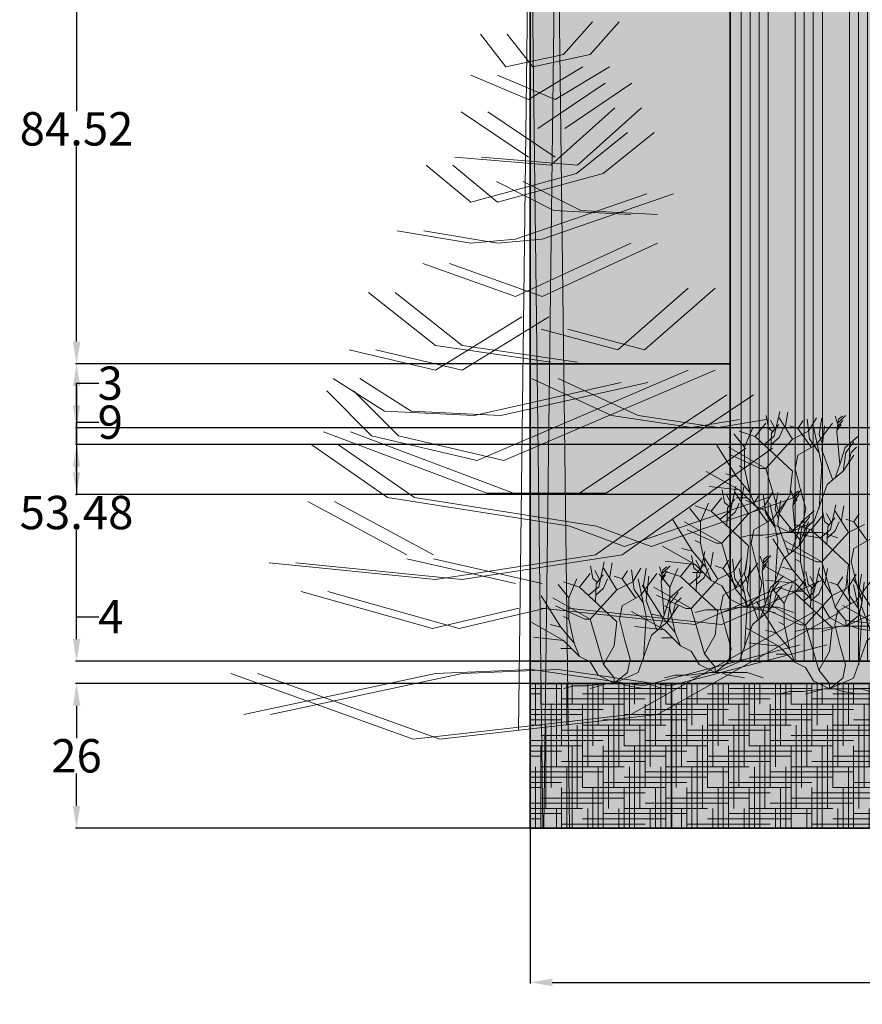
# Model space of a CAD drawing. Units: inches. Extents: x 221 to 874, y 171 to 738.
# Tile 1 of 11: x 221 to 373, y 171 to 348. Entities that reach past the tile are written whole.
import ezdxf

# ---------------------------------------------------------------- set-up
doc = ezdxf.new("R2010")
doc.units = ezdxf.units.IN
doc.header["$MEASUREMENT"] = 0
for name, color, linetype, lineweight in [('A-ANNO-DIMS', 2, 'Continuous', 18), ('A-ELEV', 7, 'Continuous', 35), ('A-ELEV-PATT', 8, 'Continuous', 13), ('L-PLNT', 3, 'Continuous', 13)]:
    doc.layers.add(name, color=color, linetype=linetype, lineweight=lineweight)
doc.styles.get("Standard").update_dxf_attribs({"font": 'arial.ttf'})
doc.dimstyles.get("Standard").update_dxf_attribs({"dimtxt": 6, "dimasz": 4, "dimexe": 0.18, "dimexo": 0.0625, "dimgap": 0.09, "dimtad": 0, "dimtih": 1, "dimtoh": 1, "dimdec": 0, "dimzin": 0, "dimdsep": 46, "dimlunit": 3, "dimtxsty": 'Standard', "dimcen": 0.09, "dimadec": 0, "dimazin": 0, "dimtfac": 1, "dimtdec": 0, "dimtofl": 0, "dimtmove": 0, "dimatfit": 3, "dimfxl": 1, "dimtolj": 1, "dimtzin": 0, "dimarcsym": 0})

# ---------------------------------------------------------------- blocks, each defined once
blk = doc.blocks.new('SHRUB-A')
for p, q in [((15.5, 17.76), (13.1, 21.6)), ((18.38, 19.2), (19.82, 21.6)), ((6.86, 16.32), (8.3, 19.68)), ((8.78, 18.24), (10.7, 20.64)), ((19.82, 16.8), (22.7, 20.64)), ((6.86, 16.32), (4.94, 18.72)), ((8.78, 18.24), (5.9, 19.2)), ((15.5, 12), (8.78, 18.24)), ((10.7, 12.48), (15.5, 17.76)), ((15.5, 17.76), (18.38, 19.2)), ((5.42, 11.04), (1.91, 16.66)), ((10.7, 12.48), (3.98, 16.32)), ((6.86, 12.48), (6.86, 16.32)), ((16.46, 14.88), (19.82, 16.8)), ((25.1, 15.36), (26.54, 17.28)), ((9.74, 12.48), (4.46, 14.88)), ((15.98, 12.48), (16.46, 14.88)), ((24.62, 12), (25.1, 15.36)), ((24.62, 12), (26.54, 14.88)), ((6.86, 12.48), (5.9, 12.96)), ((7.82, 8.16), (6.86, 12.48)), ((10.7, 12.48), (9.74, 12.48)), ((13.1, 4.32), (10.7, 12.48)), ((16.94, 8.64), (15.98, 12.48)), ((5.9, 8.64), (0, 11.96)), ((5.42, 11.04), (3.5, 11.52)), ((7.82, 8.16), (5.42, 11.04)), ((15.02, 7.68), (15.5, 12)), ((21.74, 9.6), (24.62, 12)), ((5.9, 8.64), (0.53, 9.22)), ((19.34, 2.88), (21.74, 9.6)), ((8.78, 5.76), (5.9, 8.64)), ((8.78, 5.76), (7.82, 8.16)), ((13.1, 4.32), (15.02, 7.68)), ((17.9, 5.28), (16.94, 8.64)), ((10.7, 4.8), (8.78, 5.76)), ((12.14, 2.4), (10.7, 4.8)), ((15.02, 1.92), (13.1, 4.32)), ((17.42, 2.88), (17.9, 5.28)), ((15.02, 0.96), (12.14, 2.4)), ((15.02, 0.96), (19.34, 2.88)), ((15.02, 0.96), (17.42, 2.88)), ((15.02, 0.96), (15.02, 1.92)), ((15.02, 0.96), (20.78, 0.96)), ((20.78, 0.96), (23.66, 0))]:
    blk.add_line(p, q)
blk = doc.blocks.new('GRASS-TUFT')
for p, q in [((0.58, 10.54), (1.31, 11.09)), ((0.28, 8.35), (0.58, 10.54)), ((0.83, 2.4), (0.28, 8.35)), ((1.8, 5.45), (4.12, 7.49)), ((0.83, 2.4), (1.8, 5.45)), ((0, 0), (0.83, 2.4))]:
    blk.add_line(p, q)
blk = doc.blocks.new('GRASS-SPRIG')
for p, q in [((1.44, 3.36), (0, 3.84)), ((1.44, 3.36), (2.4, 4.8)), ((3.84, 0), (1.44, 3.36))]:
    blk.add_line(p, q)
blk = doc.blocks.new('*D20')
at = {"layer": 'A-ANNO-DIMS', "color": 0, "lineweight": -2, "transparency": 16777216}
for p, q in [((313.08, 202.65), (313.08, 174.79)), ((805.08, 202.65), (805.08, 174.79)), ((317.08, 174.97), (552.27, 174.97)), ((801.08, 174.97), (565.89, 174.97))]:
    blk.add_line(p, q, dxfattribs=at)
at = {"layer": 'A-ANNO-DIMS', "color": 0, "transparency": 16777216}
for points in [[(317.08, 175.63), (317.08, 174.3), (313.08, 174.97)], [(801.08, 175.63), (801.08, 174.3), (805.08, 174.97)]]:
    blk.add_solid(points, dxfattribs=at)
at = {"layer": 'Defpoints', "color": 0, "transparency": 16777216}
for p in [(313.08, 202.72), (805.08, 202.72), (805.08, 174.97)]:
    blk.add_point(p, dxfattribs=at)
at = {"layer": 'A-ANNO-DIMS', "color": 0, "transparency": 16777216, "insert": (559.08, 174.97), "char_height": 6, "attachment_point": 5}
blk.add_mtext('\\A1;492', dxfattribs=at)
blk = doc.blocks.new('*D29')
at = {"layer": 'A-ANNO-DIMS', "color": 0, "lineweight": -2, "transparency": 16777216}
for p, q in [((313.02, 228.72), (231.36, 228.72)), ((231.54, 224.72), (231.54, 218.87)), ((231.54, 206.72), (231.54, 212.56)), ((313.02, 202.72), (231.36, 202.72))]:
    blk.add_line(p, q, dxfattribs=at)
at = {"layer": 'A-ANNO-DIMS', "color": 0, "transparency": 16777216}
for points in [[(230.88, 224.72), (232.21, 224.72), (231.54, 228.72)], [(230.88, 206.72), (232.21, 206.72), (231.54, 202.72)]]:
    blk.add_solid(points, dxfattribs=at)
at = {"layer": 'Defpoints', "color": 0, "transparency": 16777216}
for p in [(231.54, 228.72), (313.08, 228.72), (313.08, 202.72)]:
    blk.add_point(p, dxfattribs=at)
at = {"layer": 'A-ANNO-DIMS', "color": 0, "transparency": 16777216, "insert": (231.54, 215.72), "char_height": 6, "attachment_point": 5}
blk.add_mtext('\\A1;26', dxfattribs=at)
blk = doc.blocks.new('*D30')
at = {"layer": 'A-ANNO-DIMS', "color": 0, "lineweight": -2, "transparency": 16777216}
for p, q in [((231.54, 236.72), (231.54, 240.72)), ((231.54, 240.72), (235.54, 240.72)), ((313.02, 232.72), (231.36, 232.72)), ((313.02, 228.72), (231.36, 228.72)), ((231.54, 224.72), (231.54, 220.72))]:
    blk.add_line(p, q, dxfattribs=at)
at = {"layer": 'A-ANNO-DIMS', "color": 0, "transparency": 16777216}
for points in [[(230.88, 236.72), (232.21, 236.72), (231.54, 232.72)], [(230.88, 224.72), (232.21, 224.72), (231.54, 228.72)]]:
    blk.add_solid(points, dxfattribs=at)
at = {"layer": 'Defpoints', "color": 0, "transparency": 16777216}
for p in [(231.54, 232.72), (313.08, 232.72), (313.08, 228.72)]:
    blk.add_point(p, dxfattribs=at)
at = {"layer": 'A-ANNO-DIMS', "color": 0, "transparency": 16777216, "insert": (237.71, 240.72), "char_height": 6, "attachment_point": 5}
blk.add_mtext('\\A1;4', dxfattribs=at)
blk = doc.blocks.new('*D31')
at = {"layer": 'A-ANNO-DIMS', "color": 0, "lineweight": -2, "transparency": 16777216}
for p, q in [((313.02, 286.2), (231.36, 286.2)), ((231.54, 282.2), (231.54, 262.61)), ((231.54, 236.72), (231.54, 256.3)), ((313.02, 232.72), (231.36, 232.72))]:
    blk.add_line(p, q, dxfattribs=at)
at = {"layer": 'A-ANNO-DIMS', "color": 0, "transparency": 16777216}
for points in [[(230.88, 282.2), (232.21, 282.2), (231.54, 286.2)], [(230.88, 236.72), (232.21, 236.72), (231.54, 232.72)]]:
    blk.add_solid(points, dxfattribs=at)
at = {"layer": 'Defpoints', "color": 0, "transparency": 16777216}
for p in [(231.54, 286.2), (313.08, 286.2), (313.08, 232.72)]:
    blk.add_point(p, dxfattribs=at)
at = {"layer": 'A-ANNO-DIMS', "color": 0, "transparency": 16777216, "insert": (231.54, 259.46), "char_height": 6, "attachment_point": 5}
blk.add_mtext('\\A1;53.48', dxfattribs=at)
blk = doc.blocks.new('*D32')
at = {"layer": 'A-ANNO-DIMS', "color": 0, "lineweight": -2, "transparency": 16777216}
for p, q in [((313.02, 370.72), (231.36, 370.72)), ((231.54, 366.72), (231.54, 331.61)), ((231.54, 290.2), (231.54, 325.3)), ((313.02, 286.2), (231.36, 286.2))]:
    blk.add_line(p, q, dxfattribs=at)
at = {"layer": 'A-ANNO-DIMS', "color": 0, "transparency": 16777216}
for points in [[(230.88, 366.72), (232.21, 366.72), (231.54, 370.72)], [(230.88, 290.2), (232.21, 290.2), (231.54, 286.2)]]:
    blk.add_solid(points, dxfattribs=at)
at = {"layer": 'Defpoints', "color": 0, "transparency": 16777216}
for p in [(231.54, 370.72), (313.08, 370.72), (313.08, 286.2)]:
    blk.add_point(p, dxfattribs=at)
at = {"layer": 'A-ANNO-DIMS', "color": 0, "transparency": 16777216, "insert": (231.54, 328.46), "char_height": 6, "attachment_point": 5}
blk.add_mtext('\\A1;84.52', dxfattribs=at)
blk = doc.blocks.new('*D67')
at = {"layer": 'A-ANNO-DIMS', "color": 0, "lineweight": -2, "transparency": 16777216}
for p, q in [((231.54, 271.72), (231.54, 275.72)), ((231.54, 275.72), (235.54, 275.72)), ((541.02, 271.72), (231.36, 271.72)), ((231.54, 266.72), (231.54, 267.72)), ((541.02, 262.72), (231.36, 262.72))]:
    blk.add_line(p, q, dxfattribs=at)
at = {"layer": 'A-ANNO-DIMS', "color": 0, "transparency": 16777216}
for points in [[(230.88, 267.72), (232.21, 267.72), (231.54, 271.72)], [(230.88, 266.72), (232.21, 266.72), (231.54, 262.72)]]:
    blk.add_solid(points, dxfattribs=at)
at = {"layer": 'Defpoints', "color": 0, "transparency": 16777216}
for p in [(231.54, 271.72), (541.08, 271.72), (541.08, 262.72)]:
    blk.add_point(p, dxfattribs=at)
at = {"layer": 'A-ANNO-DIMS', "color": 0, "transparency": 16777216, "insert": (237.61, 275.72), "char_height": 6, "attachment_point": 5}
blk.add_mtext('\\A1;9', dxfattribs=at)
blk = doc.blocks.new('*D68')
at = {"layer": 'A-ANNO-DIMS', "color": 0, "lineweight": -2, "transparency": 16777216}
for p, q in [((231.54, 278.72), (231.54, 282.72)), ((231.54, 282.72), (235.54, 282.72)), ((541.02, 274.72), (231.36, 274.72)), ((541.02, 271.72), (231.36, 271.72)), ((231.54, 267.72), (231.54, 263.72))]:
    blk.add_line(p, q, dxfattribs=at)
at = {"layer": 'A-ANNO-DIMS', "color": 0, "transparency": 16777216}
for points in [[(230.88, 278.72), (232.21, 278.72), (231.54, 274.72)], [(230.88, 267.72), (232.21, 267.72), (231.54, 271.72)]]:
    blk.add_solid(points, dxfattribs=at)
at = {"layer": 'Defpoints', "color": 0, "transparency": 16777216}
for p in [(231.54, 274.72), (541.08, 274.72), (541.08, 271.72)]:
    blk.add_point(p, dxfattribs=at)
at = {"layer": 'A-ANNO-DIMS', "color": 0, "transparency": 16777216, "insert": (237.6, 282.72), "char_height": 6, "attachment_point": 5}
blk.add_mtext('\\A1;3', dxfattribs=at)

msp = doc.modelspace()

# ---------------------------------------------------------------- hatches: boundary and pattern name
at = {"layer": 'A-ELEV-PATT'}
h = msp.add_hatch(color=256, dxfattribs=at)
h.dxf.hatch_style = 1
h.paths.add_polyline_path([(349.0786, 286.1996), (313.0786, 286.1996), (313.0786, 232.7164), (349.0786, 232.7164)])
h.paths.add_polyline_path([(464.0786, 286.1996), (406.0786, 286.1996), (406.0786, 232.7164), (464.0786, 232.7164)])
h.paths.add_polyline_path([(541.0786, 286.1996), (493.0786, 286.1996), (493.0786, 232.7164), (541.0786, 232.7164)])
h.paths.add_polyline_path([(541.0786, 370.7164), (493.0786, 370.7164), (493.0786, 286.1996), (541.0786, 286.1996)])
h.paths.add_polyline_path([(464.0786, 370.7164), (406.0786, 370.7164), (406.0786, 286.1996), (464.0786, 286.1996)])
h.paths.add_polyline_path([(349.0786, 370.7164), (313.0786, 370.7164), (313.0786, 286.1996), (349.0786, 286.1996)])
h.paths.add_polyline_path([(349.0786, 454.7164), (313.0786, 454.7164), (313.0786, 370.7164), (349.0786, 370.7164)])
h.paths.add_polyline_path([(464.0786, 454.7164), (406.0786, 454.7164), (406.0786, 370.7164), (464.0786, 370.7164)])
h.paths.add_polyline_path([(541.0786, 418.7164), (541.0786, 454.7164), (493.0786, 454.7164), (493.0786, 370.7164), (541.0786, 370.7164)])
h.paths.add_polyline_path([(541.0786, 550.7164), (493.0786, 550.7164), (493.0786, 454.7164), (541.0786, 454.7164)])
h.paths.add_polyline_path([(464.0786, 550.7164), (406.0786, 550.7164), (406.0786, 454.7164), (464.0786, 454.7164)])
h.paths.add_polyline_path([(349.0786, 550.7164), (313.0786, 550.7164), (313.0786, 454.7164), (349.0786, 454.7164)])
h.paths.add_polyline_path([(349.0786, 586.7164), (313.0786, 586.7164), (313.0786, 550.7164), (349.0786, 550.7164)])
h.paths.add_polyline_path([(464.0786, 586.7164), (406.0786, 586.7164), (406.0786, 550.7164), (464.0786, 550.7164)])
h.paths.add_polyline_path([(541.0786, 574.7164), (541.0786, 586.7164), (493.0786, 586.7164), (493.0786, 550.7164), (541.0786, 550.7164)])
h.paths.add_polyline_path([(541.0786, 670.7164), (493.0786, 670.7164), (493.0786, 586.7164), (541.0786, 586.7164)])
h.paths.add_polyline_path([(464.0786, 670.7164), (406.0786, 670.7164), (406.0786, 586.7164), (464.0786, 586.7164)])
h.paths.add_polyline_path([(349.0786, 670.7164), (313.0786, 670.7164), (313.0786, 586.7164), (349.0786, 586.7164)])
h.paths.add_polyline_path([(406.0786, 706.7164), (313.0786, 706.7164), (313.0786, 670.7164), (349.0786, 670.7164), (406.0786, 670.7164)])
h.paths.add_polyline_path([(464.0786, 706.7164), (406.0786, 706.7164), (406.0786, 670.7164), (464.0786, 670.7164)])
h.paths.add_polyline_path([(541.0786, 706.7164), (493.0786, 706.7164), (493.0786, 688.7164), (493.0786, 670.7164), (541.0786, 670.7164)])
h.paths.add_polyline_path([(660.0786, 610.7164), (541.0786, 610.7164), (541.0786, 586.7164), (541.0786, 574.7164), (660.0786, 574.7164)])
h.paths.add_polyline_path([(781.0786, 610.7164), (660.0786, 610.7164), (660.0786, 574.7164), (769.0786, 574.7164), (781.0786, 574.7164)])
h.paths.add_polyline_path([(781.0786, 574.7164), (769.0786, 574.7164), (769.0786, 476.1199), (781.0786, 476.1199)])
h.paths.add_polyline_path([(781.0786, 476.1199), (769.0786, 476.1199), (769.0786, 457.7164), (781.0786, 457.7164)])
h.paths.add_polyline_path([(781.0786, 377.1023), (705.9097, 377.1023), (705.9097, 286.1996), (781.0786, 286.1996)])
h.paths.add_polyline_path([(741.9618, 338.8486), (756.9618, 338.8486), (756.9618, 329.8486), (741.9618, 329.8486)], flags=16)
h.paths.add_polyline_path([(648.9097, 377.1023), (598.0786, 377.1023), (598.0786, 286.1996), (648.9097, 286.1996)])
h.paths.add_polyline_path([(781.0786, 286.1996), (705.9097, 286.1996), (705.9097, 280.7164), (648.9097, 280.7164), (648.9097, 286.1996), (598.0786, 286.1996), (598.0786, 280.7164), (550.0786, 280.7164), (550.0786, 286.1996), (541.0786, 286.1996), (541.0786, 274.7164), (781.0786, 274.7164)])
h.paths.add_polyline_path([(660.0786, 562.7164), (546.3477, 562.7164), (546.3477, 457.7164), (660.0786, 457.7164)])
h = msp.add_hatch(color=256, dxfattribs=at)
h.paths.add_polyline_path([(406.0786, 670.7164), (349.0786, 670.7164), (349.0786, 454.7164), (406.0786, 454.7164)])
h.paths.add_polyline_path([(406.0786, 454.7164), (349.0786, 454.7164), (349.0786, 232.7164), (406.0786, 232.7164)])
h = msp.add_hatch(dxfattribs=at)
h.set_pattern_fill('ANSI34', color=256, scale=13, angle=45, style=0)
h.paths.add_polyline_path([(406.0786, 670.7164), (349.0786, 670.7164), (349.0786, 454.7164), (406.0786, 454.7164)])
h.paths.add_polyline_path([(406.0786, 454.7164), (349.0786, 454.7164), (349.0786, 232.7164), (406.0786, 232.7164)])
msp.add_hatch(color=256, dxfattribs=at).paths.add_polyline_path([(313.0786, 232.7164), (313.0786, 228.7164), (541.0786, 228.7164), (541.0786, 232.7164)])
h = msp.add_hatch(color=256, dxfattribs=at)
h.set_gradient(color1=(99, 100, 102), color2=(91, 91, 91), rotation=180, name='INVCURVED')
h.paths.add_polyline_path([(338.5139, 202.7164), (338.5139, 228.7164), (313.0786, 228.7164), (313.0786, 202.7164)])
h = msp.add_hatch(dxfattribs=at)
h.set_pattern_fill('HOUND', color=256, scale=15, style=0)
h.paths.add_polyline_path([(338.5139, 228.7164), (313.0786, 228.7164), (313.0786, 202.7164), (338.5139, 202.7164)])
h = msp.add_hatch(color=256, dxfattribs=at)
h.set_gradient(color1=(147, 149, 152), color2=(91, 91, 91), name='CURVED')
h.paths.add_polyline_path([(384.2386, 202.7164), (384.2386, 228.7164), (338.5139, 228.7164), (338.5139, 202.7164)])
h = msp.add_hatch(dxfattribs=at)
h.set_pattern_fill('HOUND', color=256, scale=15, style=0)
h.paths.add_polyline_path([(384.2386, 228.7164), (338.5139, 228.7164), (338.5139, 202.7164), (384.2386, 202.7164)])

# ---------------------------------------------------------------- linework, layer by layer
at = {"layer": 'A-ELEV'}
for p, q in [((313.0786, 232.7164), (313.0786, 706.7164)), ((349.0786, 232.7164), (349.0786, 670.7164)), ((313.0786, 286.1996), (349.0786, 286.1996)), ((541.0786, 232.7164), (313.0786, 232.7164)), ((313.0786, 232.7164), (313.0786, 228.7164)), ((541.0786, 228.7164), (313.0786, 228.7164)), ((313.0786, 228.7164), (313.0786, 202.7164)), ((338.5139, 228.7164), (338.5139, 202.7164)), ((805.0786, 202.7164), (313.0786, 202.7164))]:
    msp.add_line(p, q, dxfattribs=at)
at = {"layer": 'L-PLNT'}
for p, q in [((313.0656, 386.0299), (310.9947, 220.2893)), ((313.0656, 386.0299), (315.358, 202.7164)), ((317.8656, 386.0299), (315.5752, 202.7164)), ((317.8656, 386.0299), (320.158, 202.7164)), ((355.9588, 274.6734), (355.5318, 276.9424)), ((356.9968, 273.1874), (357.9728, 277.6474)), ((360.2698, 272.6584), (357.8698, 276.4984)), ((358.9498, 274.6734), (359.4378, 277.4904)), ((363.3438, 272.6394), (362.9168, 276.2384)), ((363.1498, 274.0984), (364.5898, 276.4984)), ((365.0528, 273.5004), (365.5418, 276.4734)), ((367.9218, 276.7864), (368.3488, 275.4564)), ((368.4708, 275.6124), (369.8138, 276.9424)), ((351.6298, 271.2184), (353.0698, 274.5784)), ((353.5498, 273.1384), (355.4698, 275.5384)), ((356.7528, 273.9694), (355.9588, 274.6734)), ((357.1498, 274.5174), (356.3258, 276.0824)), ((356.5088, 273.7344), (357.7898, 275.2994)), ((357.8508, 272.9524), (358.5838, 274.5954)), ((365.5498, 267.8584), (364.1098, 274.5784)), ((364.5898, 271.6984), (367.4698, 275.5384)), ((365.5498, 270.7384), (366.0298, 275.0584)), ((368.2878, 274.2824), (369.0198, 275.2994)), ((368.4098, 274.9084), (369.3258, 276.0034)), ((351.6298, 271.2184), (349.7098, 273.6184)), ((353.5498, 273.1384), (350.6698, 274.0984)), ((360.2698, 266.8984), (353.5498, 273.1384)), ((355.1048, 271.6224), (356.9968, 273.1874)), ((356.3868, 270.5264), (356.5088, 273.7344)), ((356.4478, 271.7004), (357.8508, 272.9524)), ((360.2698, 272.6584), (363.1498, 274.0984)), ((365.0528, 270.2134), (363.3438, 272.7174)), ((365.6638, 271.7004), (365.0528, 273.5004)), ((350.1898, 265.9384), (346.6748, 271.5534)), ((355.4698, 267.3784), (348.7498, 271.2184)), ((351.6298, 267.3784), (351.6298, 271.2184)), ((355.4698, 267.3784), (360.2698, 272.6584)), ((361.2298, 269.7784), (364.5898, 271.6984)), ((369.8698, 270.2584), (371.3098, 272.1784)), ((370.8298, 270.2584), (371.7898, 271.2184)), ((354.5098, 267.3784), (349.2298, 269.7784)), ((360.7498, 267.3784), (361.2298, 269.7784)), ((367.4698, 265.4584), (365.5498, 270.7384)), ((369.3898, 266.8984), (369.8698, 270.2584)), ((369.3898, 266.8984), (371.3098, 269.7784)), ((370.3498, 268.3384), (370.8298, 270.2584)), ((351.6298, 267.3784), (350.6698, 267.8584)), ((352.5898, 263.0584), (351.6298, 267.3784)), ((355.4698, 267.3784), (354.5098, 267.3784)), ((357.8698, 259.2184), (355.4698, 267.3784)), ((361.7098, 263.5384), (360.7498, 267.3784)), ((365.0698, 260.1784), (365.5498, 267.8584)), ((350.6698, 263.5384), (344.7668, 266.8594)), ((350.1898, 265.9384), (348.2698, 266.4184)), ((352.5898, 263.0584), (350.1898, 265.9384)), ((359.7898, 262.5784), (360.2698, 266.8984)), ((366.5098, 264.4984), (369.3898, 266.8984)), ((350.6698, 263.5384), (345.3018, 264.1204)), ((349.0936, 259.7609), (350.0696, 264.2209)), ((351.0466, 261.2469), (351.5346, 264.0639)), ((364.1098, 257.7784), (366.5098, 264.4984)), ((348.0556, 261.2469), (347.6286, 263.5159)), ((349.2466, 261.0909), (348.4226, 262.6559)), ((352.1098, 262.0984), (350.1898, 262.0984)), ((353.5498, 260.6584), (350.6698, 263.5384)), ((353.5498, 260.6584), (352.5898, 263.0584)), ((355.4406, 259.2129), (355.0136, 262.8119)), ((357.1496, 260.0739), (357.6386, 263.0469)), ((357.8698, 259.2184), (359.7898, 262.5784)), ((360.0186, 263.3599), (360.4456, 262.0299)), ((360.5066, 261.4819), (361.4226, 262.5769)), ((360.5676, 262.1859), (361.9106, 263.5159)), ((362.6698, 260.1784), (361.7098, 263.5384)), ((273.0956, 261.4559), (290.9246, 251.8709)), ((277.8956, 261.4559), (295.7246, 251.8709)), ((348.8496, 260.5429), (348.0556, 261.2469)), ((348.4836, 257.0999), (348.6056, 260.3079)), ((348.6056, 260.3079), (349.8866, 261.8729)), ((349.9476, 259.5259), (350.6806, 261.1689)), ((355.4698, 259.6984), (353.5498, 260.6584)), ((357.6466, 254.4319), (356.2066, 261.1519)), ((357.6466, 257.3119), (358.1266, 261.6319)), ((360.3846, 260.8559), (361.1166, 261.8729)), ((367.0768, 256.3874), (368.0528, 260.8474)), ((369.0298, 257.8734), (369.5178, 260.6904)), ((347.2016, 258.1959), (349.0936, 259.7609)), ((348.5446, 258.2739), (349.9476, 259.5259)), ((357.1496, 256.7869), (355.4406, 259.2909)), ((356.9098, 257.2984), (355.4698, 259.6984)), ((357.7606, 258.2739), (357.1496, 260.0739)), ((359.7898, 256.8184), (357.8698, 259.2184)), ((362.1898, 257.7784), (362.6698, 260.1784)), ((363.6298, 256.3384), (365.5498, 258.7384)), ((366.0388, 257.8734), (365.6118, 260.1424)), ((367.2298, 257.7174), (366.4058, 259.2824)), ((370.3498, 255.8584), (367.9498, 259.6984)), ((359.7898, 255.8584), (356.9098, 257.2984)), ((359.5666, 252.0319), (357.6466, 257.3119)), ((359.7898, 255.8584), (364.1098, 257.7784)), ((359.7898, 255.8584), (362.1898, 257.7784)), ((361.7098, 254.4184), (359.7898, 256.8184)), ((359.7898, 255.8584), (359.7898, 256.8184)), ((363.6298, 256.3384), (360.7498, 257.2984)), ((361.7098, 254.4184), (363.1498, 257.7784)), ((362.4466, 254.9119), (362.9266, 256.8319)), ((362.9266, 256.8319), (363.8866, 257.7919)), ((366.8328, 257.1694), (366.0388, 257.8734)), ((366.4668, 253.7264), (366.5888, 256.9344)), ((366.5888, 256.9344), (367.8698, 258.4994)), ((367.9308, 256.1524), (368.6638, 257.7954)), ((370.3498, 255.8584), (373.2298, 257.2984)), ((352.5898, 255.3784), (350.6698, 254.8984)), ((354.9898, 255.3784), (352.5898, 255.3784)), ((358.8298, 255.8584), (354.9898, 255.3784)), ((358.8298, 255.8584), (355.4698, 254.8984)), ((358.8298, 255.8584), (360.7498, 255.8584)), ((359.7898, 255.8584), (365.5498, 255.8584)), ((360.7498, 255.8584), (362.1898, 255.3784)), ((362.1898, 255.3784), (365.0698, 254.8984)), ((370.3498, 250.0984), (363.6298, 256.3384)), ((365.1848, 254.8224), (367.0768, 256.3874)), ((365.5498, 250.5784), (370.3498, 255.8584)), ((365.5498, 255.8584), (368.4298, 254.8984)), ((366.5278, 254.9004), (367.9308, 256.1524)), ((360.2698, 249.1384), (356.7548, 254.7534)), ((357.1666, 246.7519), (357.6466, 254.4319)), ((365.5498, 250.5784), (358.8298, 254.4184)), ((361.7098, 250.5784), (361.7098, 254.4184)), ((371.3098, 252.9784), (374.6698, 254.8984)), ((342.5149, 249.4974), (342.0879, 251.7664)), ((343.5529, 248.0114), (344.5289, 252.4714)), ((345.5059, 249.4974), (345.9939, 252.3144)), ((354.4779, 251.6104), (354.9049, 250.2804)), ((355.0269, 250.4364), (356.3699, 251.7664)), ((364.5898, 250.5784), (359.3098, 252.9784)), ((370.8298, 250.5784), (371.3098, 252.9784)), ((290.9246, 251.1339), (310.4786, 246.7099)), ((295.7246, 251.1339), (315.2786, 246.7099)), ((324.3871, 247.6064), (323.9601, 249.8754)), ((325.4251, 246.1204), (326.4011, 250.5804)), ((327.3781, 247.6064), (327.8661, 250.4234)), ((336.3501, 249.7194), (336.7771, 248.3894)), ((336.8991, 248.5454), (338.2421, 249.8754)), ((343.7059, 249.3414), (342.8819, 250.9064)), ((343.0649, 248.5584), (344.3459, 250.1234)), ((349.8999, 247.4634), (349.4729, 251.0624)), ((351.6089, 248.3244), (352.0979, 251.2974)), ((352.1059, 245.5624), (352.5859, 249.8824)), ((354.8439, 249.1064), (355.5759, 250.1234)), ((360.7498, 246.7384), (354.8468, 250.0594)), ((354.9659, 249.7324), (355.8819, 250.8274)), ((361.7098, 250.5784), (360.7498, 251.0584)), ((362.6698, 246.2584), (361.7098, 250.5784)), ((365.5498, 250.5784), (364.5898, 250.5784)), ((367.9498, 242.4184), (365.5498, 250.5784)), ((369.8698, 245.7784), (370.3498, 250.0984)), ((371.7898, 246.7384), (370.8298, 250.5784)), ((325.5781, 247.4504), (324.7541, 249.0154)), ((324.9371, 246.6674), (326.2181, 248.2324)), ((331.7721, 245.5724), (331.3451, 249.1714)), ((333.4811, 246.4334), (333.9701, 249.4064)), ((333.9781, 243.6714), (334.4581, 247.9914)), ((336.7161, 247.2154), (337.4481, 248.2324)), ((336.8381, 247.8414), (337.7541, 248.9364)), ((341.6609, 246.4464), (343.5529, 248.0114)), ((344.2066, 248.6719), (342.2866, 248.6719)), ((343.3089, 248.7934), (342.5149, 249.4974)), ((342.9429, 245.3504), (343.0649, 248.5584)), ((344.4069, 247.7764), (345.1399, 249.4194)), ((352.1059, 242.6824), (350.6659, 249.4024)), ((352.2199, 246.5244), (351.6089, 248.3244)), ((360.2698, 249.1384), (358.3498, 249.6184)), ((362.6698, 246.2584), (360.2698, 249.1384)), ((363.0868, 246.5714), (362.6598, 248.8404)), ((364.2778, 246.4154), (363.4538, 247.9804)), ((364.1248, 245.0854), (365.1008, 249.5454)), ((366.0778, 246.5714), (366.5658, 249.3884)), ((370.4718, 244.5374), (370.0448, 248.1364)), ((372.1808, 245.3984), (372.6698, 248.3714)), ((323.5331, 244.5554), (325.4251, 246.1204)), ((325.1811, 246.9024), (324.3871, 247.6064)), ((324.8151, 243.4594), (324.9371, 246.6674)), ((326.2791, 245.8854), (327.0121, 247.5284)), ((333.9781, 240.7914), (332.5381, 247.5114)), ((334.0921, 244.6334), (333.4811, 246.4334)), ((342.6846, 239.3369), (361.0886, 247.4469)), ((343.0039, 246.5244), (344.4069, 247.7764)), ((347.4846, 239.3369), (365.8886, 247.4469)), ((351.6089, 245.0374), (349.8999, 247.5414)), ((360.7498, 246.7384), (355.3818, 247.3204)), ((363.6298, 243.8584), (360.7498, 246.7384)), ((363.6298, 243.8584), (362.6698, 246.2584)), ((363.8808, 245.8674), (363.0868, 246.5714)), ((363.6368, 245.6324), (364.9178, 247.1974)), ((364.9788, 244.8504), (365.7118, 246.4934)), ((372.6778, 239.7564), (371.2378, 246.4764)), ((374.7578, 241.8364), (371.2428, 247.4514)), ((372.7498, 243.3784), (371.7898, 246.7384)), ((372.6778, 242.6364), (373.1578, 246.9564)), ((271.9456, 245.2349), (295.5246, 238.5989)), ((276.7456, 245.2349), (300.3246, 238.5989)), ((324.8761, 244.6334), (326.2791, 245.8854)), ((333.4811, 243.1464), (331.7721, 245.6504)), ((354.0259, 240.2824), (352.1059, 245.5624)), ((356.9059, 243.1624), (357.3859, 245.0824)), ((357.3859, 245.0824), (358.3459, 246.0424)), ((362.1898, 245.2984), (360.2698, 245.2984)), ((362.2328, 243.5204), (364.1248, 245.0854)), ((363.5148, 242.4244), (363.6368, 245.6324)), ((363.5758, 243.5984), (364.9788, 244.8504)), ((367.9498, 242.4184), (369.8698, 245.7784)), ((372.1808, 242.1114), (370.4718, 244.6154)), ((372.7918, 243.5984), (372.1808, 245.3984)), ((335.8981, 238.3914), (333.9781, 243.6714)), ((338.7781, 241.2714), (339.2581, 243.1914)), ((339.2581, 243.1914), (340.2181, 244.1514)), ((351.6259, 235.0024), (352.1059, 242.6824)), ((365.5498, 242.8984), (363.6298, 243.8584)), ((366.9898, 240.4984), (365.5498, 242.8984)), ((375.2378, 239.4364), (369.3348, 242.7574)), ((372.2698, 240.9784), (372.7498, 243.3784)), ((374.5978, 237.3564), (372.6778, 242.6364)), ((295.5246, 238.5989), (311.0536, 242.2859)), ((300.3246, 238.5989), (315.8536, 242.2859)), ((315.0786, 242.2859), (342.6846, 239.3369)), ((319.8786, 242.2859), (347.4846, 239.3369)), ((344.6866, 241.9519), (342.7666, 241.4719)), ((347.0866, 241.9519), (344.6866, 241.9519)), ((350.9266, 242.4319), (347.0866, 241.9519)), ((350.9266, 242.4319), (347.5666, 241.4719)), ((350.9266, 242.4319), (352.8466, 242.4319)), ((352.8466, 242.4319), (354.2866, 241.9519)), ((354.2866, 241.9519), (357.1666, 241.4719)), ((369.8698, 240.0184), (367.9498, 242.4184)), ((369.8698, 239.0584), (374.1898, 240.9784)), ((369.8698, 239.0584), (372.2698, 240.9784)), ((333.4981, 233.1114), (333.9781, 240.7914)), ((368.9098, 239.0584), (365.0698, 238.5784)), ((368.9098, 239.0584), (365.5498, 238.0984)), ((369.8698, 239.0584), (366.9898, 240.4984)), ((368.9098, 239.0584), (370.8298, 239.0584)), ((375.2378, 239.4364), (369.8698, 240.0184)), ((369.8698, 239.0584), (369.8698, 240.0184)), ((369.8698, 239.0584), (375.6298, 239.0584)), ((370.8298, 239.0584), (372.2698, 238.5784)), ((372.1978, 232.0764), (372.6778, 239.7564)), ((362.6698, 238.5784), (360.7498, 238.0984)), ((365.0698, 238.5784), (362.6698, 238.5784)), ((372.2698, 238.5784), (375.1498, 238.0984)), ((338.6659, 236.9224), (336.7459, 236.9224)), ((320.5381, 235.0314), (318.6181, 235.0314)), ((359.2378, 233.9964), (357.3178, 233.9964)), ((339.1459, 230.2024), (337.2259, 229.7224)), ((341.5459, 230.2024), (339.1459, 230.2024)), ((345.3859, 230.6824), (341.5459, 230.2024)), ((345.3859, 230.6824), (342.0259, 229.7224)), ((345.3859, 230.6824), (347.3059, 230.6824)), ((347.3059, 230.6824), (348.7459, 230.2024)), ((348.7459, 230.2024), (351.6259, 229.7224)), ((327.2581, 228.7914), (323.4181, 228.3114)), ((327.2581, 228.7914), (323.8981, 227.8314)), ((327.2581, 228.7914), (329.1781, 228.7914)), ((329.1781, 228.7914), (330.6181, 228.3114)), ((321.0181, 228.3114), (319.0981, 227.8314)), ((323.4181, 228.3114), (321.0181, 228.3114)), ((330.6181, 228.3114), (333.4981, 227.8314)), ((359.7178, 227.2764), (357.7978, 226.7964)), ((362.1178, 227.2764), (359.7178, 227.2764)), ((365.9578, 227.7564), (362.1178, 227.2764)), ((365.9578, 227.7564), (362.5978, 226.7964)), ((365.9578, 227.7564), (367.8778, 227.7564)), ((367.8778, 227.7564), (369.3178, 227.2764)), ((369.3178, 227.2764), (372.1978, 226.7964))]:
    msp.add_line(p, q, dxfattribs=at)
for points in [[(324.2806, 347.7209), (319.1046, 341.8219), (308.7526, 339.6099), (304.1516, 345.5089)], [(329.0806, 347.7209), (323.9046, 341.8219), (313.5526, 339.6099), (308.9516, 345.5089)], [(302.4266, 338.1359), (312.7786, 333.7119), (322.5556, 339.6099)], [(307.2266, 338.1359), (317.5786, 333.7119), (327.3556, 339.6099)], [(314.5036, 328.5509), (326.5816, 336.6609)], [(319.3036, 328.5509), (331.3816, 336.6609)], [(299.5506, 323.3899), (316.8046, 321.9149), (328.3066, 332.2369)], [(300.7006, 331.4999), (312.7786, 323.3899)], [(304.3506, 323.3899), (321.6046, 321.9149), (333.1066, 332.2369)], [(305.5006, 331.4999), (317.5786, 323.3899)], [(294.3746, 321.9149), (302.4266, 315.2789), (321.4056, 320.4399), (330.6076, 327.8129)], [(299.1746, 321.9149), (307.2266, 315.2789), (326.2056, 320.4399), (335.4076, 327.8129)], [(307.0276, 318.9659), (317.3796, 313.8049), (331.1826, 313.0669)], [(311.8276, 318.9659), (322.1796, 313.8049), (335.9826, 313.0669)], [(289.1986, 310.1179), (302.4266, 307.9059), (310.4786, 308.6429), (334.0576, 316.7539)], [(293.9986, 310.1179), (307.2266, 307.9059), (315.2786, 308.6429), (338.8576, 316.7539)], [(293.7996, 304.2199), (310.4786, 298.3209), (331.1826, 307.9059)], [(298.5996, 304.2199), (315.2786, 298.3209), (335.9826, 307.9059)], [(315.0786, 292.4229), (328.8816, 288.7359), (341.5346, 299.7959)], [(319.8786, 292.4229), (333.6816, 288.7359), (346.3346, 299.7959)], [(284.0226, 299.0579), (296.1006, 289.4729), (316.8046, 286.5239)], [(288.8226, 299.0579), (300.9006, 289.4729), (321.6046, 286.5239)], [(280.5716, 288.7359), (296.1006, 285.0499), (311.6286, 294.6349)], [(285.3716, 288.7359), (300.9006, 285.0499), (316.4286, 294.6349)], [(276.5466, 281.3629), (284.5976, 273.2529), (303.5766, 268.8289), (341.5346, 285.0499)], [(277.6966, 283.5749), (286.8986, 277.6769), (303.0016, 276.9389), (329.4566, 282.8379)], [(281.3466, 281.3629), (289.3976, 273.2529), (308.3766, 268.8289), (346.3346, 285.0499)], [(282.4966, 283.5749), (291.6986, 277.6769), (307.8016, 276.9389), (334.2566, 282.8379)], [(313.3536, 283.5749), (327.7316, 276.9389), (342.1096, 274.7269), (350.7366, 276.2019)], [(318.1536, 283.5749), (332.5316, 276.9389), (346.9096, 274.7269), (355.5366, 276.2019)], [(275.9706, 273.9899), (305.3016, 262.9309), (321.9806, 262.9309), (348.4356, 280.6259)], [(280.7706, 273.9899), (310.1016, 262.9309), (326.7806, 262.9309), (353.2356, 280.6259)], [(266.1946, 250.3959), (296.1006, 247.4469), (324.8556, 251.8709), (351.8866, 271.0409)], [(270.9946, 250.3959), (300.9006, 247.4469), (329.6556, 251.8709), (356.6866, 271.0409)], [(273.6706, 271.7779), (287.4736, 262.1929), (320.2546, 257.0319), (330.0316, 253.3459), (355.9126, 262.1929)], [(278.4706, 271.7779), (292.2736, 262.1929), (325.0546, 257.0319), (334.8316, 253.3459), (360.7126, 262.1929)], [(259.2926, 230.4889), (292.0746, 218.6919), (331.1826, 223.1159), (363.9636, 241.5489)], [(264.0926, 230.4889), (296.8746, 218.6919), (335.9826, 223.1159), (368.7636, 241.5489)], [(261.5936, 223.1159), (296.1006, 230.4889), (313.3536, 231.2259), (333.4826, 228.2769), (361.6636, 235.6499)], [(266.3936, 223.1159), (300.9006, 230.4889), (318.1536, 231.2259), (338.2826, 228.2769), (366.4636, 235.6499)]]:
    msp.add_lwpolyline(points, dxfattribs=at)

# ---------------------------------------------------------------- block references
for name, p in [('GRASS-TUFT', (367.9502, 265.698)), ('GRASS-SPRIG', (359.7902, 271.218)), ('SHRUB-A', (336.8639, 241.4716)), ('GRASS-SPRIG', (351.887, 257.7916)), ('GRASS-TUFT', (360.047, 252.2716)), ('GRASS-SPRIG', (369.8702, 254.418)), ('GRASS-TUFT', (354.5063, 240.522)), ('SHRUB-A', (331.3231, 229.722)), ('GRASS-TUFT', (336.3785, 238.6311)), ('GRASS-SPRIG', (346.3463, 246.042)), ('SHRUB-A', (313.1954, 227.8311)), ('GRASS-SPRIG', (328.2185, 244.1511)), ('SHRUB-A', (351.895, 226.796)), ('GRASS-SPRIG', (366.9182, 243.116))]:
    msp.add_blockref(name, p, dxfattribs=at)

# ---------------------------------------------------------------- dimensions: what is measured, and where the dimension line sits
at = {"layer": 'A-ANNO-DIMS'}
for base, p1, p2, override, picture, middle in [((231.5426, 370.7164), (313.0786, 286.1996), (313.0786, 370.7164), {"dimdec": 2, "dimlfac": 1, "dimrnd": 0, "dimzin": 0, "dimdsep": 46, "dimlunit": 2}, '*D32', (231.5426, 328.458)), ((231.5426, 286.1996), (313.0786, 232.7164), (313.0786, 286.1996), {"dimdec": 2, "dimlfac": 1, "dimrnd": 0, "dimzin": 0, "dimdsep": 46, "dimlunit": 2}, '*D31', (231.5426, 259.458)), ((231.5426, 274.7164), (541.0786, 271.7164), (541.0786, 274.7164), {"dimdec": 0, "dimlfac": 1, "dimrnd": 0, "dimzin": 0, "dimdsep": 46, "dimlunit": 2}, '*D68', (237.5972, 282.7164)), ((231.5426, 271.7164), (541.0786, 262.7164), (541.0786, 271.7164), {"dimdec": 0, "dimlfac": 1, "dimrnd": 0, "dimzin": 0, "dimdsep": 46, "dimlunit": 2}, '*D67', (237.6053, 275.7164)), ((231.5426, 232.7164), (313.0786, 228.7164), (313.0786, 232.7164), {"dimdec": 0, "dimlfac": 1, "dimrnd": 0, "dimzin": 0, "dimdsep": 46, "dimlunit": 2}, '*D30', (237.7077, 240.7164)), ((231.5426, 228.7164), (313.0786, 202.7164), (313.0786, 228.7164), {"dimdec": 0, "dimlfac": 1, "dimrnd": 0, "dimzin": 0, "dimdsep": 46, "dimlunit": 2}, '*D29', (231.5426, 215.7164))]:
    dim = msp.add_linear_dim(base=base, p1=p1, p2=p2, angle=90, dimstyle='Standard', override=override, dxfattribs=at)
    dim.commit()
    dim.dimension.update_dxf_attribs({"geometry": picture, "text_midpoint": middle})
dim = msp.add_linear_dim(base=(805.0786, 174.9664), p1=(313.0786, 202.7164), p2=(805.0786, 202.7164), dimstyle='Standard', override={"dimdec": 0, "dimlfac": 1, "dimrnd": 0, "dimzin": 0, "dimdsep": 46, "dimlunit": 2}, dxfattribs=at)
dim.commit()
dim.dimension.update_dxf_attribs({"geometry": '*D20', "text_midpoint": (559.0786, 174.9664)})

doc.saveas('drawing.dxf')
